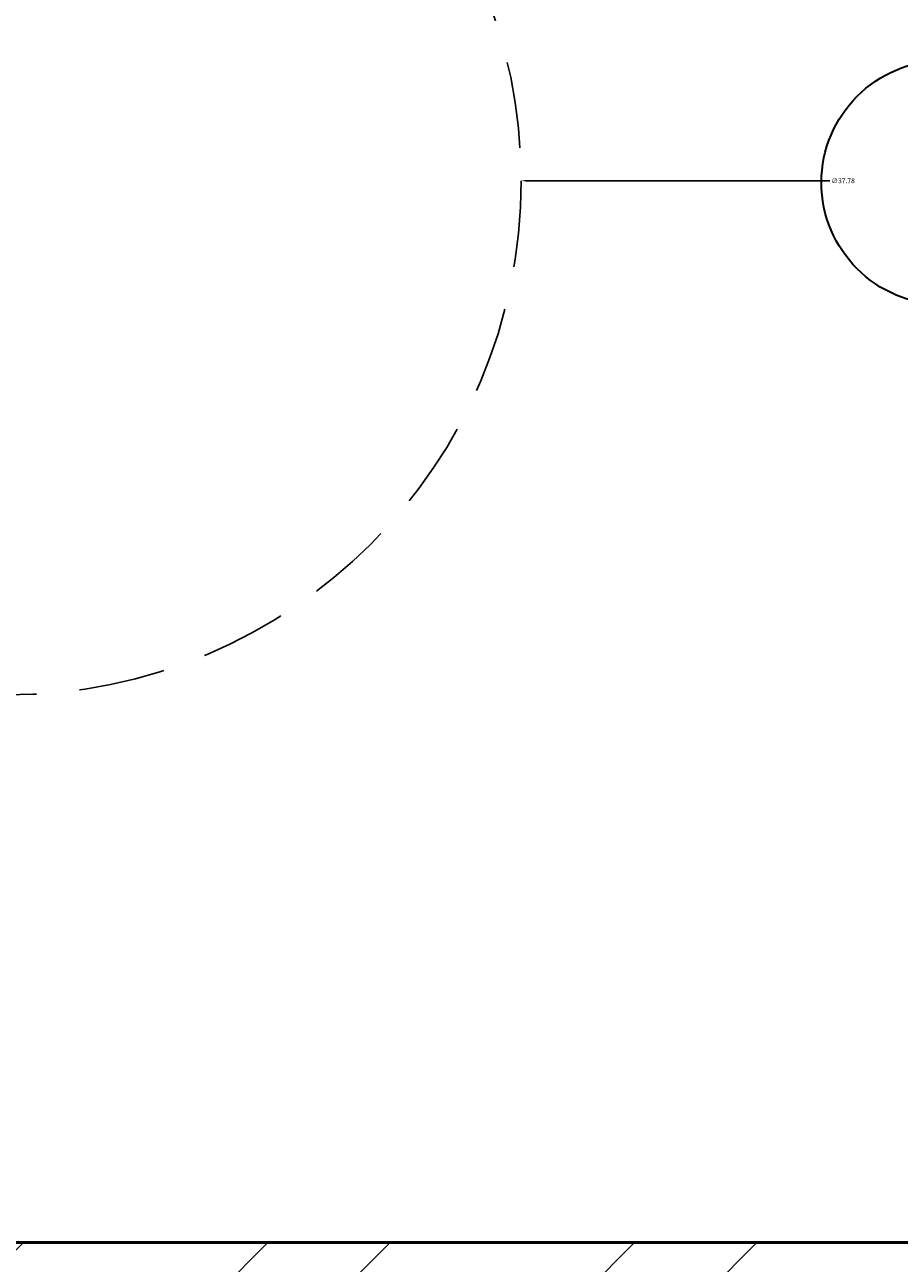
# Model space of a CAD drawing. Units: inches. Extents: x 2812 to 3051, y 1398 to 1659.
# Tile 52 of 65: x 2911 to 2944, y 1559 to 1605. Entities that reach past the tile are written whole.
import ezdxf

# ---------------------------------------------------------------- set-up
doc = ezdxf.new("R2010")
doc.units = ezdxf.units.IN
doc.linetypes.add('HIDDEN2', pattern=[4.7625, 3.175, -1.5875])
for name, color, linetype, lineweight in [('A-ANNO-DIMS', 2, 'Continuous', 18), ('P-SANR-PIPE', 4, 'Continuous', 35), ('S-CONC', 7, 'Continuous', 50), ('S-CONC-HIDN', 8, 'HIDDEN2', 25), ('S-CONC-PATT', 8, 'Continuous', 18)]:
    doc.layers.add(name, color=color, linetype=linetype, lineweight=lineweight)
doc.styles.get("Standard").update_dxf_attribs({"font": 'arial.ttf'})
doc.dimstyles.get("Standard").update_dxf_attribs({"dimtxt": 0.18, "dimasz": 0.18, "dimexe": 0.18, "dimexo": 0.0625, "dimgap": 0.09, "dimtad": 0, "dimtih": 1, "dimtoh": 1, "dimdec": 4, "dimzin": 0, "dimdsep": 46, "dimtxsty": 'Standard', "dimcen": 0.09, "dimadec": 0, "dimazin": 0, "dimtfac": 1, "dimtdec": 4, "dimtofl": 0, "dimtmove": 0, "dimatfit": 3, "dimfxl": 1, "dimtolj": 1, "dimtzin": 0, "dimarcsym": 0})

# ---------------------------------------------------------------- blocks, each defined once
blk = doc.blocks.new('*D84')
at = {"layer": 'A-ANNO-DIMS', "color": 0, "lineweight": -2, "transparency": 16777216}
for p, q in [((2910.652, 1598.82), (2910.832, 1598.82)), ((2910.742, 1598.73), (2910.742, 1598.91)), ((2940.963, 1598.82), (2929.81, 1598.82))]:
    blk.add_line(p, q, dxfattribs=at)
at = {"layer": 'A-ANNO-DIMS', "color": 0, "transparency": 16777216}
blk.add_solid([(2929.81, 1598.85), (2929.81, 1598.79), (2929.63, 1598.82)], dxfattribs=at)
at = {"layer": 'Defpoints', "color": 0, "transparency": 16777216}
for p in [(2891.853, 1598.82), (2929.63, 1598.82)]:
    blk.add_point(p, dxfattribs=at)
at = {"layer": 'A-ANNO-DIMS', "color": 0, "transparency": 16777216, "insert": (2941.455, 1598.82), "char_height": 0.18, "attachment_point": 5}
blk.add_mtext('\\A1;∅37.78', dxfattribs=at)

msp = doc.modelspace()

# ---------------------------------------------------------------- hatches: boundary and pattern name
at = {"layer": 'S-CONC-PATT'}
h = msp.add_hatch(dxfattribs=at)
h.set_pattern_fill('ANSI32', color=256)
h.paths.add_polyline_path([(3027.3849, 1646.82), (2835.3849, 1646.82), (2835.3849, 1603.2296), (2844.3849, 1603.2296), (2844.3849, 1637.82), (3018.3849, 1637.82), (3018.3849, 1602.5441), (3027.3849, 1602.5441)])
h.paths.add_polyline_path([(2844.3849, 1594.2296), (2835.3849, 1594.2296), (2835.3849, 1550.82), (3027.3849, 1550.82), (3027.3849, 1593.5441), (3018.3849, 1593.5441), (3018.3849, 1559.82), (2844.3849, 1559.82)])
h.paths.add_polyline_path([(2844.3849, 1482.0354), (2835.3849, 1482.0354), (2835.3849, 1463.4959), (2844.3849, 1463.4959)])
h.paths.add_polyline_path([(2844.3849, 1461.4959), (2835.3849, 1461.4959), (2835.3849, 1416.0354), (2844.3849, 1416.0354)])
h.paths.add_polyline_path([(3027.3849, 1482.0354), (3018.3849, 1482.0354), (3018.3849, 1463.2854), (3027.3849, 1463.2854)])
h.paths.add_polyline_path([(3027.3849, 1461.2854), (3018.3849, 1461.2854), (3018.3849, 1416.0354), (3027.3849, 1416.0354)])
h.paths.add_polyline_path([(2961.3849, 1448.4738), (2952.3849, 1448.4738), (2952.3849, 1416.0354), (2961.3849, 1416.0354)])
h.paths.add_polyline_path([(2961.3849, 1462.3026), (2952.3849, 1462.3026), (2952.3849, 1450.4738), (2961.3849, 1450.4738)])
h.paths.add_polyline_path([(2961.3849, 1472.0354), (2952.3849, 1472.0354), (2952.3849, 1462.3026), (2961.3849, 1462.3026)])

# ---------------------------------------------------------------- linework, layer by layer
at = {"layer": 'P-SANR-PIPE'}
msp.add_circle((2945.1467, 1598.7541), 4.4867, dxfattribs=at)
at = {"layer": 'S-CONC'}
msp.add_line((2844.3849, 1559.82), (3018.3849, 1559.82), dxfattribs=at)
at = {"layer": 'S-CONC-HIDN'}
msp.add_circle((2910.7415, 1598.82), 18.8884, dxfattribs=at)

# ---------------------------------------------------------------- dimensions: what is measured, and where the dimension line sits
at = {"layer": 'A-ANNO-DIMS'}
dim = msp.add_diameter_dim_2p(p1=(2891.8531, 1598.8199), p2=(2929.6299, 1598.82), dimstyle='Standard', override={"dimdec": 2, "dimlfac": 1, "dimrnd": 0, "dimzin": 0, "dimdsep": 46, "dimlunit": 2}, dxfattribs=at)
dim.commit()
dim.dimension.update_dxf_attribs({"geometry": '*D84', "text_midpoint": (2940.963, 1598.82), "dimtype": 163})

doc.saveas('drawing.dxf')
